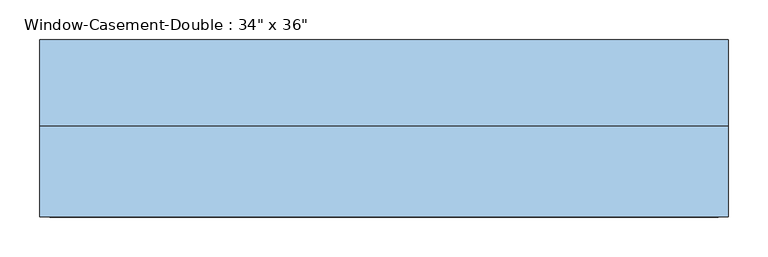
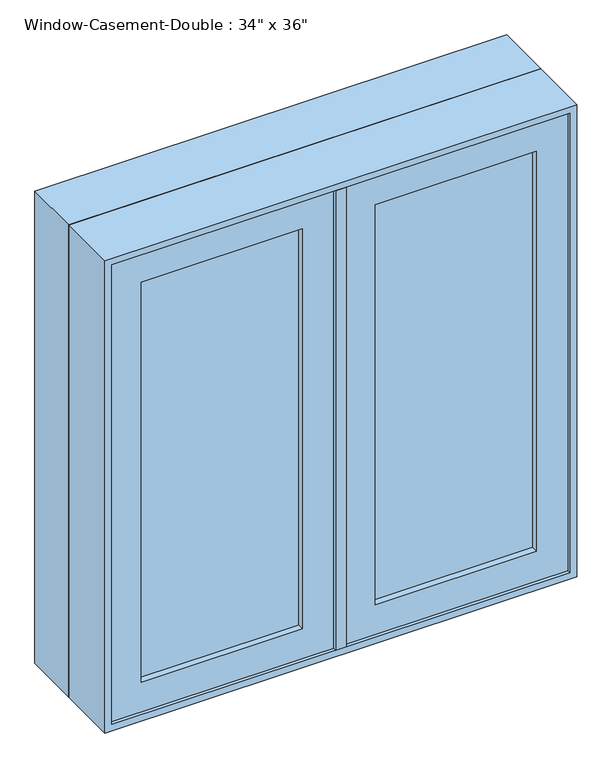
"""IFC4 building model written with IfcOpenShell, lengths in millimetres: window geometry."""

from ifc_helpers import new_model, si_unit, frame, origin, place, context, project, spatial, polyline, outline, extrude, faceted_brep, source, transform, mapped, element, save


def window_99681c7d(model_context):
    return source(origin(), model_context, "Body", "SolidModel", [
        faceted_brep([(9.525, -120.65, 1816.1), (9.525, -69.85, 1816.1), (-9.525, -69.85, 1816.1), (-9.525, -120.65, 1816.1), (9.525, -120.65, 927.1), (-9.525, -120.65, 927.1), (-9.525, -69.85, 927.1), (9.525, -69.85, 927.1), (-9.525, -69.85, 1797.05), (-9.525, -69.85, 946.15), (-30.1625, -69.85, 1797.05), (-30.1625, -69.85, 946.15), (-30.1625, -6.35, 1797.05), (-30.1625, -6.35, 946.15), (30.1625, -6.35, 1797.05), (30.1625, -6.35, 946.15), (30.1625, -69.85, 1797.05), (30.1625, -69.85, 946.15), (9.525, -69.85, 1797.05), (9.525, -69.85, 946.15)], [[[0, 1, 2, 3]], [[4, 5, 6, 7]], [[3, 5, 4, 0]], [[2, 8, 9, 6, 5, 3]], [[8, 10, 11, 9]], [[10, 12, 13, 11]], [[12, 14, 15, 13]], [[14, 16, 17, 15]], [[16, 18, 19, 17]], [[0, 4, 7, 19, 18, 1]], [[8, 2, 1, 18]], [[19, 7, 6, 9]], [[9, 11, 13, 15, 17, 19]], [[18, 16, 14, 12, 10, 8]]]),
        extrude(outline(polyline([(-66.675, -101.6), (-361.95, -101.6), (-361.95, -95.25), (-66.675, -95.25), (-66.675, -101.6)])), frame((0.0, 0.0, 984.25), z_axis=(0.0, 0.0, 1.0), x_axis=(1.0, 0.0, 0.0)), (0.0, 0.0, 1.0), 774.7),
        extrude(outline(polyline([(-361.95, -82.55), (-66.675, -82.55), (-66.675, -88.9), (-361.95, -88.9), (-361.95, -82.55)])), frame((0.0, 0.0, 984.25), z_axis=(0.0, 0.0, 1.0), x_axis=(1.0, 0.0, 0.0)), (0.0, 0.0, 1.0), 774.7),
        extrude(outline(polyline([(361.95, -101.6), (66.675, -101.6), (66.675, -95.25), (361.95, -95.25), (361.95, -101.6)])), frame((0.0, 0.0, 984.25), z_axis=(0.0, 0.0, 1.0), x_axis=(1.0, 0.0, 0.0)), (0.0, 0.0, 1.0), 774.7),
        extrude(outline(polyline([(66.675, -82.55), (361.95, -82.55), (361.95, -88.9), (66.675, -88.9), (66.675, -82.55)])), frame((0.0, 0.0, 984.25), z_axis=(0.0, 0.0, 1.0), x_axis=(1.0, 0.0, 0.0)), (0.0, 0.0, 1.0), 774.7),
        extrude(outline(polyline([(1816.1, -9.525), (1816.1, -419.1), (927.1, -419.1), (927.1, -9.525), (1816.1, -9.525)]), holes=[polyline([(1758.95, -361.95), (1758.95, -66.675), (984.25, -66.675), (984.25, -361.95), (1758.95, -361.95)])]), frame((0.0, -114.3, 0.0), z_axis=(0.0, 1.0, 0.0), x_axis=(0.0, 0.0, 1.0)), (0.0, 0.0, 1.0), 44.45),
        extrude(outline(polyline([(927.1, 9.525), (927.1, 419.1), (1816.1, 419.1), (1816.1, 9.525), (927.1, 9.525)]), holes=[polyline([(984.25, 361.95), (984.25, 66.675), (1758.95, 66.675), (1758.95, 361.95), (984.25, 361.95)])]), frame((0.0, -114.3, 0.0), z_axis=(0.0, 1.0, 0.0), x_axis=(0.0, 0.0, 1.0)), (0.0, 0.0, 1.0), 44.45),
        extrude(outline(polyline([(1828.8, -431.8), (914.4, -431.8), (914.4, 431.8), (1828.8, 431.8), (1828.8, -431.8)]), holes=[polyline([(1809.75, 412.75), (933.45, 412.75), (933.45, -412.75), (1809.75, -412.75), (1809.75, 412.75)])]), frame((0.0, -6.35, 0.0), z_axis=(0.0, 1.0, 0.0), x_axis=(0.0, 0.0, 1.0)), (0.0, 0.0, 1.0), 107.95),
        faceted_brep([(400.05, -69.85, 1797.05), (-400.05, -69.85, 1797.05), (-400.05, -6.35, 1797.05), (400.05, -6.35, 1797.05), (419.1, -120.65, 1816.1), (-419.1, -120.65, 1816.1), (-419.1, -69.85, 1816.1), (419.1, -69.85, 1816.1), (431.8, -6.35, 1828.8), (-431.8, -6.35, 1828.8), (-431.8, -120.65, 1828.8), (431.8, -120.65, 1828.8), (-400.05, -69.85, 946.15), (-400.05, -6.35, 946.15), (-419.1, -120.65, 927.1), (-419.1, -69.85, 927.1), (-431.8, -6.35, 914.4), (-431.8, -120.65, 914.4), (400.05, -69.85, 946.15), (400.05, -6.35, 946.15), (419.1, -120.65, 927.1), (419.1, -69.85, 927.1), (431.8, -6.35, 914.4), (431.8, -120.65, 914.4)], [[[0, 1, 2, 3]], [[4, 5, 6, 7]], [[8, 9, 10, 11]], [[1, 12, 13, 2]], [[5, 14, 15, 6]], [[9, 16, 17, 10]], [[12, 18, 19, 13]], [[14, 20, 21, 15]], [[16, 22, 23, 17]], [[9, 8, 22, 16], [3, 2, 13, 19]], [[18, 0, 3, 19]], [[7, 6, 15, 21], [1, 0, 18, 12]], [[20, 4, 7, 21]], [[22, 8, 11, 23]], [[11, 10, 17, 23], [5, 4, 20, 14]]]),
    ])


if __name__ == "__main__":
    model = new_model("IFC4")
    model_context = context("Model", 3, world=origin())
    ifc_project = project(units=[si_unit("LENGTHUNIT", "METRE", prefix="MILLI")], contexts=[model_context])
    site = spatial("IfcSite", under=ifc_project)
    building = spatial("IfcBuilding", under=site)
    placement = place(None, origin())
    window_shape = window_99681c7d(model_context)
    element("IfcWindow", 1, ObjectType="Window-Casement-Double : 34\" x 36\"", at=placement, inside=building, context=model_context, shape_type="MappedRepresentation", body=[
        mapped(window_shape, transform((0.0, 0.0, 0.0), x_axis=(1.0, 0.0, 0.0), y_axis=(0.0, 1.0, 0.0), z_axis=(0.0, 0.0, 1.0))),
    ])
    save(model, "model.ifc")

# Revit data of these elements
# Type "Window-Casement-Double : 34\" x 36\""
#   Type Mark = "14"
#   Fire Rating = "0.5h"
#   Assembly Code = "B2020100"
#   Analytic Construction = "Double glazing - domestic"
#   Frame Extension [instance default] = 0' - 0 1/4"
#   Window Inset [instance default] = 0' - 0"
#   Wall Thickness [instance default] = 0' - 6"
#   Interior Wall Closure [instance default] = 0' - 2 1/4"
#   Half Width = 1' - 5"
#   Visual Light Transmittance = 0.81
#   Thermal Resistance (R) = 1.8146 (h·ft²·°F)/BTU
#   Solar Heat Gain Coefficient = 0.76
#   Rough Width = 2' - 10 1/2"
#   Rough Height = 3' - 0 1/2"
#   Height = 3' - 0"
#   Heat Transfer Coefficient (U) = 0.5511 BTU/(h·ft²·°F)
#   Exterior Wall Closure [instance default] = 0' - 1 1/4"
#   Extension Jamb [instance default] = 0' - 2 1/4"
#   Default Sill Height = 3' - 0"
#   Width = 2' - 10"
#   Define Thermal Properties by = 0
#   Muntin Visibility = yes
#   Interior Trim Visibility [instance default] = yes
#   Exterior Trim Visibility [instance default] = yes
#   Extension Jamb Visibility [instance default] = yes
#   Interior Trim Material = Wood - Stained
#   Muntin Pattern = Muntin Pattern_2x2 : Muntin Pattern_2x2
#   Interior Trim = Trim-Window-Interior-Flat : Picture Frame
#   Interior Frame Material = Wood - Stained
#   Glass Panel Material = Glass
#   Exterior Trim Material = Clad - White
#   Exterior Trim = Trim-Window-Exterior-Flat : with Sill
#   Exterior Frame Material = Clad - White
#   Wall Closure = (empty or 0)
# Element 1 (IfcWindow, "Window-Casement-Double : 34\" x 36\"")
#   Wall Thickness = 0' - 8"
#   Extension Jamb = 0' - 4 1/4"
#   Materials on its faces: "Wood - Stained", "Glass", "Clad - White"
# Materials
#   "Wood - Stained": class "Wood", colour RGB 224 178 126, transparency 0, Cost = 0
#   "Glass": class "Glass", colour RGB 0 128 192, transparency 0.75, Description = "Soda Lime Glass", Cost = 0
#   "Clad - White": class "Wood", colour RGB 242 242 238, transparency 0, Cost = 0
